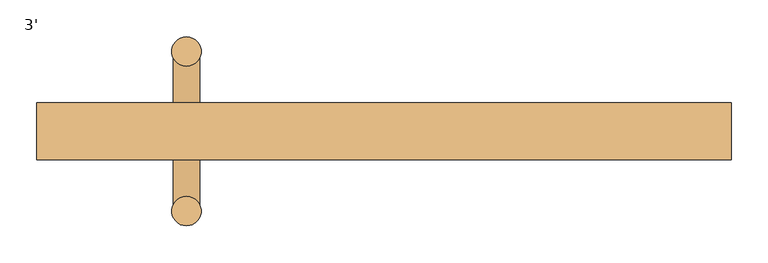
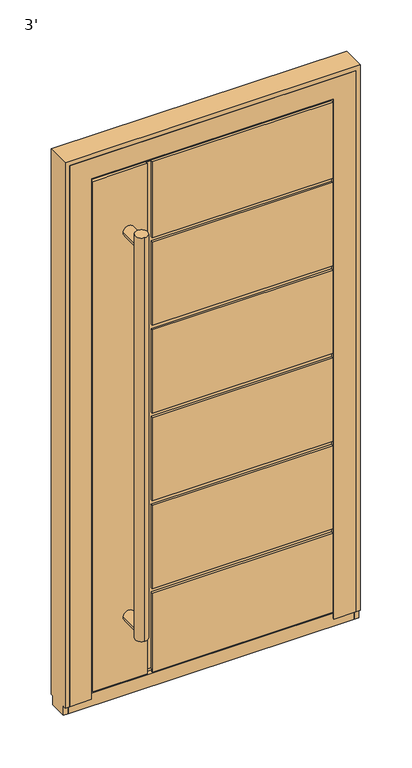
"""IFC4 building model written with IfcOpenShell, lengths in millimetres: door geometry, 3'."""

from ifc_helpers import new_model, si_unit, point, frame, frame_2d, origin, place, context, project, spatial, circle_curve, trimmed, segment, composite_curve, outline, extrude, faceted_brep, source, transform, mapped, element, save


def door_3_abbf6f65(model_context):
    return source(origin(), model_context, "Body", "SolidModel", [
        extrude(outline(composite_curve([segment(trimmed(circle_curve(frame_2d((-268.65, -52.7003001)), 20.0), [point((-268.65, -32.7003001))], [point((-268.65, -72.7003001))], False, "CARTESIAN"), True, "CONTINUOUS"), segment(trimmed(circle_curve(frame_2d((-268.65, -52.7003001)), 20.0), [point((-268.65, -72.7003001))], [point((-268.65, -32.7003001))], False, "CARTESIAN"), True, "CONTINUOUS")], self_intersect=False)), frame((0.0, 0.0, 210.0000003), z_axis=(0.0, 0.0, 1.0), x_axis=(1.0, 0.0, 0.0)), (0.0, 0.0, 1.0), 1363.8),
        extrude(outline(composite_curve([segment(trimmed(circle_curve(frame_2d((-268.65, 164.3003001)), 20.0), [point((-268.65, 184.3003001))], [point((-268.65, 144.3003001))], False, "CARTESIAN"), True, "CONTINUOUS"), segment(trimmed(circle_curve(frame_2d((-268.65, 164.3003001)), 20.0), [point((-268.65, 144.3003001))], [point((-268.65, 184.3003001))], False, "CARTESIAN"), True, "CONTINUOUS")], self_intersect=False)), frame((0.0, 0.0, 210.0000003), z_axis=(0.0, 0.0, 1.0), x_axis=(1.0, 0.0, 0.0)), (0.0, 0.0, 1.0), 1363.8),
        extrude(outline(composite_curve([segment(trimmed(circle_curve(frame_2d((241.9000003, -268.65)), 18.0), [point((241.9000003, -286.65))], [point((241.9000003, -250.65))], False, "CARTESIAN"), True, "CONTINUOUS"), segment(trimmed(circle_curve(frame_2d((241.9000003, -268.65)), 18.0), [point((241.9000003, -250.65))], [point((241.9000003, -286.65))], False, "CARTESIAN"), True, "CONTINUOUS")], self_intersect=False)), frame((0.0, -52.7, 0.0), z_axis=(0.0, 1.0, 0.0), x_axis=(0.0, 0.0, 1.0)), (0.0, 0.0, 1.0), 217.0),
        extrude(outline(composite_curve([segment(trimmed(circle_curve(frame_2d((1541.9000003, -268.65)), 18.0), [point((1541.9000003, -286.65))], [point((1541.9000003, -250.65))], False, "CARTESIAN"), True, "CONTINUOUS"), segment(trimmed(circle_curve(frame_2d((1541.9000003, -268.65)), 18.0), [point((1541.9000003, -250.65))], [point((1541.9000003, -286.65))], False, "CARTESIAN"), True, "CONTINUOUS")], self_intersect=False)), frame((0.0, -52.7, 0.0), z_axis=(0.0, 1.0, 0.0), x_axis=(0.0, 0.0, 1.0)), (0.0, 0.0, 1.0), 217.0),
        faceted_brep([(-193.65, 24.3, 306.466667), (-193.65, 24.3, 587.9333337), (383.65, 24.3, 587.9333337), (383.65, 24.3, 602.9333337), (-193.65, 24.3, 602.9333337), (-193.65, 24.3, 884.4000004), (383.65, 24.3, 884.4000004), (383.65, 24.3, 899.4000004), (-193.65, 24.3, 899.4000004), (-193.65, 24.3, 1180.866667), (383.65, 24.3, 1180.866667), (383.65, 24.3, 1195.866667), (-193.65, 24.3, 1195.866667), (-193.65, 24.3, 1477.3333337), (383.65, 24.3, 1477.3333337), (383.65, 24.3, 1492.3333337), (-193.65, 24.3, 1492.3333337), (-193.65, 24.3, 1748.8000003), (-208.65, 24.3, 1748.8000003), (-208.65, 24.3, 35.0), (-193.65, 24.3, 35.0), (-193.65, 24.3, 291.466667), (383.65, 24.3, 291.466667), (383.65, 24.3, 306.466667), (-193.65, 17.3, 306.466667), (-193.65, 17.3, 587.9333337), (383.65, 17.3, 587.9333337), (383.65, 26.3002302, 1748.8000003), (383.65, 17.3, 1748.8000003), (383.65, 17.3, 1492.3333337), (383.65, 17.3, 1477.3333337), (383.65, 17.3, 1195.866667), (383.65, 17.3, 1180.866667), (383.65, 17.3, 899.4000004), (383.65, 17.3, 884.4000004), (383.65, 17.3, 602.9333337), (383.65, 17.3, 306.466667), (383.65, 17.3, 291.466667), (383.65, 17.3, 24.0), (383.65, 19.2979528, 24.0), (383.65, 19.2979528, 35.0), (383.65, 26.3002302, 35.0), (-193.65, 17.3, 602.9333337), (-193.65, 17.3, 884.4000004), (-193.65, 17.3, 899.4000004), (-193.65, 17.3, 1180.866667), (-208.65, 17.3, 1748.8000003), (-208.65, 17.3, 24.0), (-208.65, 19.2979528, 24.0), (-208.65, 19.2979528, 35.0), (-193.65, 19.2979528, 35.0), (-383.65, 19.2979528, 35.0), (-383.65, 26.3002302, 35.0), (-193.65, 17.3, 291.466667), (-193.65, 19.2979528, 24.0), (-193.65, 17.3, 24.0), (-383.65, 19.2979528, 24.0), (-383.65, 17.3, 24.0), (-383.65, 17.3, 1748.8000003), (-193.65, 17.3, 1477.3333337), (-193.65, 17.3, 1195.866667), (-193.65, 17.3, 1748.8000003), (-193.65, 17.3, 1492.3333337), (408.65, 94.3, 10.0000003), (408.65, 91.3, 10.0000003), (-193.65, 91.3, 10.0000003), (-193.65, 94.3, 10.0000003), (-408.65, 91.3, 10.0000003), (-408.65, 94.3, 10.0000003), (-208.65, 94.3, 10.0000003), (-208.65, 91.3, 10.0000003), (408.65, 94.3, 291.466667), (408.65, 91.3, 291.466667), (408.65, 94.3, 306.466667), (408.65, 94.3, 587.9333337), (408.65, 91.3, 587.9333337), (408.65, 91.3, 306.466667), (408.65, 94.3, 899.4000004), (408.65, 94.3, 1180.866667), (408.65, 91.3, 1180.866667), (408.65, 91.3, 899.4000004), (408.65, 94.3, 602.9333337), (408.65, 94.3, 884.4000004), (408.65, 91.3, 884.4000004), (408.65, 91.3, 602.9333337), (408.65, 94.3, 1195.866667), (408.65, 94.3, 1477.3333337), (408.65, 91.3, 1477.3333337), (408.65, 91.3, 1195.866667), (408.65, 94.3, 1773.8000003), (408.65, 91.3, 1773.8000003), (408.65, 91.3, 1492.3333337), (408.65, 94.3, 1492.3333337), (393.15, 91.3, 291.466667), (393.15, 91.3, 25.5), (-193.65, 91.3, 25.5), (393.15, 91.3, 587.9333337), (393.15, 91.3, 306.466667), (393.15, 91.3, 1180.866667), (393.15, 91.3, 899.4000004), (393.15, 91.3, 884.4000004), (393.15, 91.3, 602.9333337), (393.15, 91.3, 1477.3333337), (393.15, 91.3, 1195.866667), (-193.65, 91.3, 1773.8000003), (-193.65, 91.3, 1758.3000003), (393.15, 91.3, 1758.3000003), (393.15, 91.3, 1492.3333337), (-393.15, 91.3, 25.5), (-393.15, 91.3, 1758.3000003), (-208.65, 91.3, 1758.3000003), (-208.65, 91.3, 1773.8000003), (-408.65, 91.3, 1773.8000003), (-208.65, 91.3, 25.5), (-193.65, 87.3, 291.466667), (-193.65, 94.3, 291.466667), (-193.65, 87.3, 25.5), (-193.65, 94.3, 306.466667), (-193.65, 94.3, 587.9333337), (-193.65, 94.3, 899.4000004), (-193.65, 94.3, 1180.866667), (-193.65, 94.3, 602.9333337), (-193.65, 94.3, 884.4000004), (-193.65, 94.3, 1195.866667), (-193.65, 94.3, 1477.3333337), (-193.65, 94.3, 1492.3333337), (-193.65, 94.3, 1773.8000003), (-408.65, 94.3, 1773.8000003), (-208.65, 94.3, 1773.8000003), (-208.65, 87.3, 1758.3000003), (-208.65, 87.3, 25.5), (-383.65, 26.3002302, 1748.8000003), (393.15, 26.3002302, 1758.3000003), (-393.15, 26.3002302, 1758.3000003), (-393.15, 26.3002302, 25.5), (393.15, 26.3002302, 25.5), (393.15, 87.3, 291.466667), (393.15, 87.3, 306.466667), (393.15, 87.3, 587.9333337), (393.15, 87.3, 602.9333337), (393.15, 87.3, 884.4000004), (393.15, 87.3, 899.4000004), (393.15, 87.3, 1180.866667), (393.15, 87.3, 1195.866667), (393.15, 87.3, 1477.3333337), (393.15, 87.3, 1492.3333337), (-193.65, 87.3, 1477.3333337), (-193.65, 87.3, 1195.866667), (-193.65, 87.3, 1180.866667), (-193.65, 87.3, 899.4000004), (-193.65, 87.3, 884.4000004), (-193.65, 87.3, 602.9333337), (-193.65, 87.3, 587.9333337), (-193.65, 87.3, 306.466667), (-193.65, 87.3, 1758.3000003), (-193.65, 87.3, 1492.3333337)], [[[0, 1, 2, 3, 4, 5, 6, 7, 8, 9, 10, 11, 12, 13, 14, 15, 16, 17, 18, 19, 20, 21, 22, 23]], [[1, 0, 24, 25]], [[1, 25, 26, 2]], [[27, 28, 29, 15, 14, 30, 31, 11, 10, 32, 33, 7, 6, 34, 35, 3, 2, 26, 36, 23, 22, 37, 38, 39, 40, 41]], [[42, 4, 3, 35]], [[5, 4, 42, 43]], [[5, 43, 34, 6]], [[44, 8, 7, 33]], [[9, 8, 44, 45]], [[19, 18, 46, 47, 48, 49]], [[41, 40, 50, 20, 19, 49, 51, 52]], [[53, 21, 20, 50, 54, 55]], [[21, 53, 37, 22]], [[24, 0, 23, 36]], [[40, 39, 54, 50]], [[56, 51, 49, 48]], [[39, 38, 55, 54]], [[57, 56, 48, 47]], [[33, 32, 45, 44]], [[35, 34, 43, 42]], [[36, 26, 25, 24]], [[55, 38, 37, 53]], [[58, 57, 47, 46]], [[31, 30, 59, 60]], [[28, 61, 62, 29]], [[63, 64, 65, 66]], [[67, 68, 69, 70]], [[64, 63, 71, 72]], [[73, 74, 75, 76]], [[77, 78, 79, 80]], [[81, 82, 83, 84]], [[85, 86, 87, 88]], [[89, 90, 91, 92]], [[65, 64, 72, 93, 94, 95]], [[76, 75, 96, 97]], [[80, 79, 98, 99]], [[84, 83, 100, 101]], [[88, 87, 102, 103]], [[90, 104, 105, 106, 107, 91]], [[108, 109, 110, 111, 112, 67, 70, 113]], [[114, 115, 66, 65, 95, 116]], [[63, 66, 115, 71]], [[74, 73, 117, 118]], [[78, 77, 119, 120]], [[82, 81, 121, 122]], [[86, 85, 123, 124]], [[89, 92, 125, 126]], [[68, 127, 128, 69]], [[68, 67, 112, 127]], [[129, 130, 113, 70, 69, 128, 111, 110]], [[58, 131, 52, 51, 56, 57]], [[132, 133, 134, 135], [131, 27, 41, 52]], [[106, 132, 135, 94, 93, 136, 137, 97, 96, 138, 139, 101, 100, 140, 141, 99, 98, 142, 143, 103, 102, 144, 145, 107]], [[94, 135, 134, 108, 113, 130, 116, 95]], [[133, 109, 108, 134]], [[146, 147, 143, 142, 148, 149, 141, 140, 150, 151, 139, 138, 152, 153, 137, 136, 114, 116, 130, 129, 154, 155, 145, 144]], [[149, 148, 120, 119]], [[149, 119, 77, 80, 99, 141]], [[122, 150, 140, 100, 83, 82]], [[151, 150, 122, 121]], [[151, 121, 81, 84, 101, 139]], [[118, 152, 138, 96, 75, 74]], [[153, 152, 118, 117]], [[153, 117, 73, 76, 97, 137]], [[115, 114, 136, 93, 72, 71]], [[9, 45, 32, 10]], [[60, 12, 11, 31]], [[13, 12, 60, 59]], [[13, 59, 30, 14]], [[62, 16, 15, 29]], [[16, 62, 61, 17]], [[124, 146, 144, 102, 87, 86]], [[125, 155, 154, 105, 104, 126]], [[120, 148, 142, 98, 79, 78]], [[147, 123, 85, 88, 103, 143]], [[147, 146, 124, 123]], [[155, 125, 92, 91, 107, 145]], [[90, 89, 126, 104]], [[127, 112, 111, 128]], [[132, 106, 105, 154, 129, 110, 109, 133]], [[27, 131, 58, 46, 18, 17, 61, 28]]]),
        faceted_brep([(-457.2, 94.3, 0.0), (-412.7, 94.3, 0.0), (-412.7, 85.3, 0.0), (-457.2, 85.2997571, 0.0), (-403.2, 21.8000042, 0.0), (-387.7, 21.8000042, 0.0), (-387.7, 17.3, 0.0), (-457.2, 17.3, 0.0), (-457.2, 26.3, 0.0), (-403.2, 26.3, 0.0), (457.2, 17.3, 0.0), (387.7, 17.3, 0.0), (387.7, 21.8000042, 0.0), (403.2, 21.8000042, 0.0), (403.2, 26.3, 0.0), (457.2, 26.3, 0.0), (412.7, 85.3, 0.0), (412.7, 94.3, 0.0), (457.2, 94.3, 0.0), (457.2, 85.2997571, 0.0), (-457.2, 17.3, 1828.8), (-457.2, 94.3, 1828.8), (-457.2, 85.2997571, -30.0), (-457.2, 26.3, -30.0), (457.2, 94.3, 1828.8), (412.7, 94.3, 1784.3), (-412.7, 94.3, 1784.3), (457.2, 17.3, 1828.8), (457.2, 26.3, -30.0), (457.2, 85.2997571, -30.0), (-387.7, 17.3, 1759.3), (387.7, 17.3, 1759.3), (-403.2, 85.3, 1774.8), (-403.2, 21.8000042, 1774.8), (-403.2, 26.3, 14.5), (-403.2, 85.3, 14.5), (403.2, 85.3, 1774.8), (403.2, 21.8000042, 1774.8), (403.2, 85.3, 14.5), (403.2, 26.3, 14.5), (-412.7, 85.3, 1784.3), (412.7, 85.3, 1784.3), (387.7, 21.8000042, 1759.3), (-387.7, 21.8000042, 1759.3)], [[[0, 1, 2, 3]], [[4, 5, 6, 7, 8, 9]], [[10, 11, 12, 13, 14, 15]], [[16, 17, 18, 19]], [[7, 20, 21, 0, 3, 22, 23, 8]], [[1, 0, 21, 24, 18, 17, 25, 26]], [[21, 20, 27, 24]], [[18, 24, 27, 10, 15, 28, 29, 19]], [[7, 6, 30, 31, 11, 10, 27, 20]], [[32, 33, 4, 9, 34, 35]], [[33, 32, 36, 37]], [[37, 36, 38, 39, 14, 13]], [[40, 2, 1, 26]], [[16, 19, 29, 22, 3, 2, 40, 41], [36, 32, 35, 38]], [[5, 4, 33, 37, 13, 12, 42, 43]], [[6, 5, 43, 30]], [[26, 25, 41, 40]], [[31, 30, 43, 42]], [[17, 16, 41, 25]], [[12, 11, 31, 42]], [[23, 28, 15, 14, 39, 34, 9, 8]], [[38, 35, 34, 39]], [[23, 22, 29, 28]]]),
        faceted_brep([(-457.2, 85.3, -30.0), (-457.2, 26.3, -30.0), (-472.2, 26.3, -30.0), (-472.2, 85.3, -30.0), (-457.2, 94.3, 1828.8), (-457.2, 17.3, 1828.8), (-457.2, 17.3, 0.0), (-457.2, 26.3, 0.0), (-457.2, 85.3, 0.0), (-457.2, 94.3, 0.0), (472.2, 26.3, 0.0), (457.2, 26.3, 0.0), (457.2, 26.3, -30.0), (472.2, 26.3, -30.0), (-472.2, 26.3, 0.0), (-472.2, 17.3, 1843.8), (-472.2, 94.3, 1843.8), (-472.2, 94.3, 0.0), (-472.2, 85.3, 0.0), (-472.2, 17.3, 0.0), (457.2, 85.3, 0.0), (472.2, 85.3, 0.0), (472.2, 85.3, -30.0), (457.2, 85.3, -30.0), (457.2, 17.3, 1828.8), (457.2, 94.3, 1828.8), (457.2, 94.3, 0.0), (457.2, 17.3, 0.0), (472.2, 94.3, 1843.8), (472.2, 94.3, 0.0), (472.2, 17.3, 0.0), (472.2, 17.3, 1843.8)], [[[0, 1, 2, 3]], [[4, 5, 6, 7, 1, 0, 8, 9]], [[10, 11, 12, 13]], [[7, 14, 2, 1]], [[15, 16, 17, 18, 3, 2, 14, 19]], [[20, 21, 22, 23]], [[18, 8, 0, 3]], [[24, 25, 26, 20, 23, 12, 11, 27]], [[25, 4, 9, 17, 16, 28, 29, 26]], [[21, 20, 26, 29]], [[8, 18, 17, 9]], [[22, 13, 12, 23]], [[11, 10, 30, 27]], [[14, 7, 6, 19]], [[5, 24, 27, 30, 31, 15, 19, 6]], [[28, 31, 30, 10, 13, 22, 21, 29]], [[5, 4, 25, 24]], [[16, 15, 31, 28]]]),
    ])


if __name__ == "__main__":
    model = new_model("IFC4")
    model_context = context("Model", 3, world=origin())
    ifc_project = project(units=[si_unit("LENGTHUNIT", "METRE", prefix="MILLI")], contexts=[model_context])
    site = spatial("IfcSite", under=ifc_project)
    building = spatial("IfcBuilding", under=site)
    placement = place(None, origin())
    door_3_shape = door_3_abbf6f65(model_context)
    element("IfcDoor", 1, ObjectType="3'", at=placement, inside=building, context=model_context, shape_type="MappedRepresentation", body=[
        mapped(door_3_shape, transform((0.0, 0.0, 0.0), x_axis=(1.0, 0.0, 0.0), y_axis=(0.0, 1.0, 0.0), z_axis=(0.0, 0.0, 1.0))),
    ])
    save(model, "model.ifc")

# Revit data of these elements
# Type "3'"
#   Type Mark = "41"
#   Water resistance = "up to Class E900, EN 12208:2001"
#   Uniclass2015Version = "v1.21"
#   Uniclass2015Reference = "Ss_25_30_20_30"
#   Uniclass2015Description = "Frame and door leaf system"
#   URL = "www.aluprof.com"
#   Type IFC Predefined Type = "USERDEFINED"
#   Right-hand / Left-hand door [instance default] = ""
#   Resistance to wind load = "up to Class C5/B5, EN 12210:2001"
#   Insert type = "ST"
#   Hardware [instance default] = ""
#   Product page = "https://aluprof.com/en/architects/offer/window-and-door-systems/panel-doors#visualisation"
#   Operation = "SinglePanelOutwardOpening"
#   Opening type = "Outward"
#   NBSReference = "25-50-20/125"
#   NBSDescription = "Frame and door leaf system"
#   Important = "The actual acceptable construction dimensions are dependent on the selection of profiles and hardware, glazing type, construction weight and the construction’s operating conditions. These should be determined by a suitably qualified person, and using ALUPROF’s calculation software"
#   IfcExportType = "USERDEFINED"
#   IfcExportAs = "IfcDoorType"
#   Handle type [instance default] = ""
#   Manufacturer = "ALUPROF SA"
#   Export Type to IFC As = "IfcDoorType"
#   Door sill type [instance default] = ""
#   Description = "External single-leaf panel door outward opening"
#   Model = "MB-86 ST Panel Door AD07"
#   Content of the recyclate in the material = "69.2%"
#   COBie.Type.WarrantyDurationParts = ""
#   COBie.Type.Name = ""
#   COBie.Type.Manufacturer = "ALUPROF SA"
#   COBie.Space.Name = ""
#   COBie.Floor.Name = ""
#   COBie.Facility.Name = ""
#   COBie.CreatedOn = ""
#   COBie.Component.WarrantyStartDate = ""
#   COBie.Component.Name = "MB-86 ST Panel Door AD07"
#   Burglar resistance = "RC2"
#   Air permeability = "up to Class 4, EN 12207:2001"
#   Width of the active leaf = 2' - 8.17717"
#   Placement in wall = 0' - 0.7874"
#   Thickness = 0' - 3.0315"
#   Height of the opening sash = 5' - 9.44094"
#   Handle Offset = 3' - 5.33858"
#   Rough Height = 6' - 2.40945"
#   Rough Width = 3' - 1.1811"
#   Height = 6' - 0"
#   Width = 3' - 0"
#   Construction depth = 0' - 3.0315"
#   Clear opening width = 2' - 3.94882"
#   Clear opening height = 5' - 8.47638"
#   Height of the array = 0' - 11.08136"
#   Schedule No. [instance default] = 1
#   Handrail [instance default] = yes
#   IsExternal = yes
#   Handle [instance default] = no
#   Door closer [instance default] = no
#   Function = 1
#   COBie.Type = yes
#   COBie = yes
#   Access control [instance default] = no
#   Panel = element 371215
#   Wall Closure = (empty or 0)
